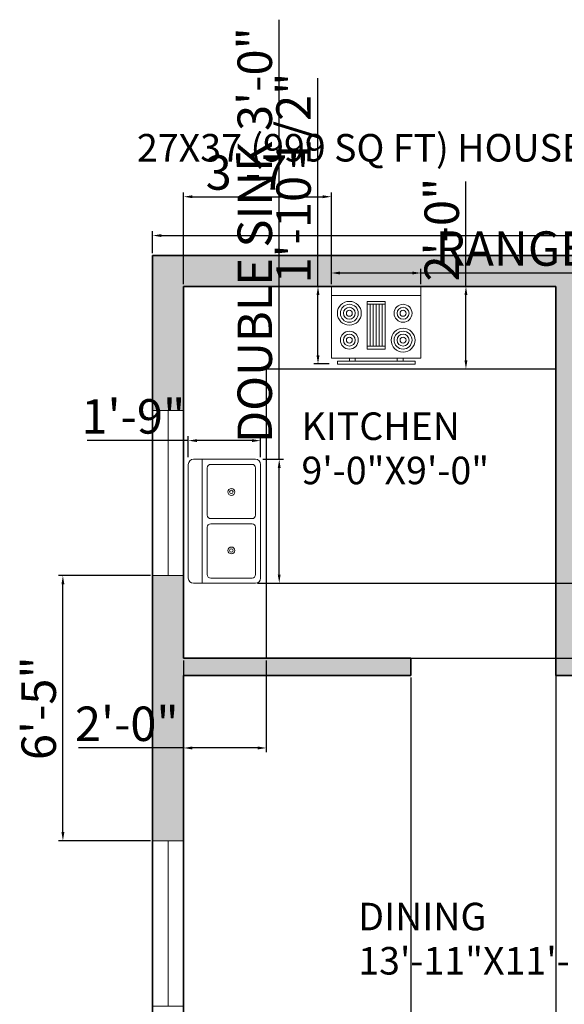
# Model space of a CAD drawing. Units: inches. Extents: x 3647 to 4124, y 1633 to 2205.
# Tile 2 of 3: x 3675 to 3833, y 1919 to 2205. Entities that reach past the tile are written whole.
import ezdxf

# ---------------------------------------------------------------- set-up
doc = ezdxf.new("R2010")
doc.units = ezdxf.units.IN
for name, color, linetype, lineweight in [('A-ANNO-DIMS', 2, 'Continuous', 18), ('A-ANNO-TEXT', 3, 'Continuous', 25), ('A-AREA-IDEN', 3, 'Continuous', 18), ('A-EQPM', 8, 'Continuous', 18), ('A-FLOR-CASE', 32, 'Continuous', 25), ('A-FLOR-FIXT', 9, 'Continuous', 18), ('WALL', 42, 'Continuous', 35), ('WINDOW', 4, 'Continuous', 18)]:
    doc.layers.add(name, color=color, linetype=linetype, lineweight=lineweight)
doc.layers.add('A-WALL-PATT', color=18, linetype='Continuous', lineweight=13, true_color=0x000000)
doc.styles.get("Standard").update_dxf_attribs({"font": 'arial.ttf'})
doc.dimstyles.new('ISO-25', dxfattribs={"dimtxt": 10, "dimasz": 2.5, "dimexe": 1.25, "dimexo": 0.625, "dimtad": 1, "dimdec": 1, "dimlunit": 3, "dimtxsty": 'Standard', "dimcen": 2.5, "dimadec": 0, "dimazin": 0, "dimtfac": 1, "dimtdec": 1, "dimtmove": 0, "dimatfit": 3, "dimfxl": 1, "dimarcsym": 0})

# ---------------------------------------------------------------- blocks, each defined once
blk = doc.blocks.new('Range-Oven - 30 in top')
for p, q in [((0, -3), (30, -3)), ((12, -6), (18, -6)), ((13, -20), (13, -6)), ((14, -6), (14, -20)), ((15, -20), (15, -6)), ((16, -6), (16, -20)), ((17, -20), (17, -6)), ((18, -20), (12, -20)), ((6, -24), (6, -25)), ((8, -25), (8, -24)), ((22, -25), (22, -24)), ((24, -24), (24, -25))]:
    blk.add_line(p, q)
for points in [[(0, -24), (0, 0), (30, 0), (30, -24)], [(12, -21), (12, -5), (18, -5), (18, -21)], [(2, -26), (2, -25), (28, -25), (28, -26)]]:
    blk.add_lwpolyline(points, close=True)
for centre, radius in [((6, -9), 4), ((6, -9), 3), ((24, -9), 3), ((6, -9), 2), ((6, -9), 1), ((24, -9), 2), ((24, -9), 1), ((6, -18), 3), ((6, -18), 2), ((24, -18), 4), ((24, -18), 3), ((24, -18), 2), ((6, -18), 1), ((24, -18), 1)]:
    blk.add_circle(centre, radius)
blk = doc.blocks.new('Sink-double - 36 in top')
for p, q in [((-18, -4), (18, -4)), ((-0.75, -18.5), (-0.75, -6.5)), ((0.75, -6.5), (0.75, -18.5))]:
    blk.add_line(p, q)
for points in [[(-16.5, 0), (16.5, 0)], [(-18, -19.5), (-18, -1.5)], [(18, -1.5), (18, -19.5)], [(-15.5, -5.5), (-1.75, -5.5)], [(1.75, -5.5), (15.5, -5.5)], [(-16.5, -18.5), (-16.5, -6.5)], [(16.5, -6.5), (16.5, -18.5)], [(-1.75, -19.5), (-15.5, -19.5)], [(15.5, -19.5), (1.75, -19.5)], [(16.5, -21), (-16.5, -21)]]:
    blk.add_lwpolyline(points)
for centre, radius in [((-8.5, -12.5), 1), ((-8.5, -12.5), 0.5), ((8.5, -12.5), 1), ((8.5, -12.5), 0.5)]:
    blk.add_circle(centre, radius)
for centre, radius, start, end in [((-16.5, -1.5), 1.5, 90, 180), ((16.5, -1.5), 1.5, 0, 90), ((-15.5, -6.5), 1, 90, 180), ((-1.75, -6.5), 1, 0, 90), ((1.75, -6.5), 1, 90, 180), ((15.5, -6.5), 1, 0, 90), ((-16.5, -19.5), 1.5, 180, 270), ((-15.5, -18.5), 1, 180, 270), ((-1.75, -18.5), 1, 270, 0), ((1.75, -18.5), 1, 180, 270), ((15.5, -18.5), 1, 270, 0), ((16.5, -19.5), 1.5, 270, 0)]:
    blk.add_arc(centre, radius, start, end)
blk = doc.blocks.new('*D11')
at = {"layer": 'A-ANNO-DIMS', "color": 0, "lineweight": -2, "transparency": 16777216}
for p, q in [((3713.71, 2136.91), (3713.71, 2143.3)), ((3716.21, 2142.05), (4035.21, 2142.05)), ((4037.71, 2136.91), (4037.71, 2143.3))]:
    blk.add_line(p, q, dxfattribs=at)
at = {"layer": 'A-ANNO-DIMS', "color": 0, "transparency": 16777216}
for points in [[(3716.21, 2142.46), (3716.21, 2141.63), (3713.71, 2142.05)], [(4035.21, 2142.46), (4035.21, 2141.63), (4037.71, 2142.05)]]:
    blk.add_solid(points, dxfattribs=at)
at = {"layer": 'Defpoints', "color": 0, "transparency": 16777216}
for p in [(4037.71, 2142.05), (3713.71, 2136.28), (4037.71, 2136.28)]:
    blk.add_point(p, dxfattribs=at)
at = {"layer": 'A-ANNO-DIMS', "color": 0, "transparency": 16777216, "insert": (3875.71, 2147.69), "char_height": 10, "attachment_point": 5}
blk.add_mtext("27'", dxfattribs=at)
blk = doc.blocks.new('WIN-48IN')
for p, q in [((9, 48), (0, 48)), ((4.5, 48), (4.5, 0)), ((9, 0), (0, 0))]:
    blk.add_line(p, q)
blk = doc.blocks.new('*D21')
at = {"layer": 'A-ANNO-DIMS', "color": 0, "lineweight": -2, "transparency": 16777216}
for p, q in [((3765.61, 2127.91), (3765.61, 2132.43)), ((3768.11, 2131.18), (3789.11, 2131.18)), ((3791.61, 2127.91), (3791.61, 2132.43)), ((3791.61, 2131.18), (3874.98, 2131.18))]:
    blk.add_line(p, q, dxfattribs=at)
at = {"layer": 'A-ANNO-DIMS', "color": 0, "transparency": 16777216}
for points in [[(3768.11, 2131.6), (3768.11, 2130.76), (3765.61, 2131.18)], [(3789.11, 2131.6), (3789.11, 2130.76), (3791.61, 2131.18)]]:
    blk.add_solid(points, dxfattribs=at)
at = {"layer": 'Defpoints', "color": 0, "transparency": 16777216}
for p in [(3791.61, 2131.18), (3765.61, 2127.28), (3791.61, 2127.28)]:
    blk.add_point(p, dxfattribs=at)
at = {"layer": 'A-ANNO-DIMS', "color": 0, "transparency": 16777216, "insert": (3834.55, 2136.98), "char_height": 10, "attachment_point": 5}
blk.add_mtext('RANGE 2\'-2"', dxfattribs=at)
blk = doc.blocks.new('*D22')
at = {"layer": 'A-ANNO-DIMS', "color": 0, "lineweight": -2, "transparency": 16777216}
for p, q in [((3761.71, 2127.28), (3761.71, 2187.74)), ((3764.98, 2127.28), (3760.46, 2127.28)), ((3761.71, 2107.25), (3761.71, 2124.78)), ((3764.98, 2104.75), (3760.46, 2104.75))]:
    blk.add_line(p, q, dxfattribs=at)
at = {"layer": 'A-ANNO-DIMS', "color": 0, "transparency": 16777216}
for points in [[(3761.29, 2124.78), (3762.13, 2124.78), (3761.71, 2127.28)], [(3761.29, 2107.25), (3762.13, 2107.25), (3761.71, 2104.75)]]:
    blk.add_solid(points, dxfattribs=at)
at = {"layer": 'Defpoints', "color": 0, "transparency": 16777216}
for p in [(3761.71, 2127.28), (3765.61, 2127.28), (3765.61, 2104.75)]:
    blk.add_point(p, dxfattribs=at)
at = {"layer": 'A-ANNO-DIMS', "color": 0, "transparency": 16777216, "insert": (3755.91, 2158.76), "char_height": 10, "attachment_point": 5, "rotation": 90}
blk.add_mtext('1\'-10 1/2"', dxfattribs=at)
blk = doc.blocks.new('*D23')
at = {"layer": 'A-ANNO-DIMS', "color": 0, "lineweight": -2, "transparency": 16777216}
for p, q in [((3750.46, 2077.09), (3750.46, 2204.75)), ((3745.68, 2077.09), (3751.71, 2077.09)), ((3750.46, 2043.59), (3750.46, 2074.59)), ((3745.68, 2041.09), (3751.71, 2041.09))]:
    blk.add_line(p, q, dxfattribs=at)
at = {"layer": 'A-ANNO-DIMS', "color": 0, "transparency": 16777216}
for points in [[(3750.04, 2074.59), (3750.87, 2074.59), (3750.46, 2077.09)], [(3750.04, 2043.59), (3750.87, 2043.59), (3750.46, 2041.09)]]:
    blk.add_solid(points, dxfattribs=at)
at = {"layer": 'Defpoints', "color": 0, "transparency": 16777216}
for p in [(3745.06, 2077.09), (3750.46, 2077.09), (3745.06, 2041.09)]:
    blk.add_point(p, dxfattribs=at)
at = {"layer": 'A-ANNO-DIMS', "color": 0, "transparency": 16777216, "insert": (3744.65, 2142.17), "char_height": 10, "attachment_point": 5, "rotation": 90}
blk.add_mtext('DOUBLE SINK 3\'-0"', dxfattribs=at)
blk = doc.blocks.new('*D24')
at = {"layer": 'A-ANNO-DIMS', "color": 0, "lineweight": -2, "transparency": 16777216}
for p, q in [((3724.06, 2082.49), (3694.66, 2082.49)), ((3724.06, 2077.72), (3724.06, 2083.74)), ((3742.56, 2082.49), (3726.56, 2082.49)), ((3745.06, 2077.72), (3745.06, 2083.74))]:
    blk.add_line(p, q, dxfattribs=at)
at = {"layer": 'A-ANNO-DIMS', "color": 0, "transparency": 16777216}
for points in [[(3726.56, 2082.91), (3726.56, 2082.08), (3724.06, 2082.49)], [(3742.56, 2082.91), (3742.56, 2082.08), (3745.06, 2082.49)]]:
    blk.add_solid(points, dxfattribs=at)
at = {"layer": 'Defpoints', "color": 0, "transparency": 16777216}
for p in [(3724.06, 2082.49), (3724.06, 2077.09), (3745.06, 2077.09)]:
    blk.add_point(p, dxfattribs=at)
at = {"layer": 'A-ANNO-DIMS', "color": 0, "transparency": 16777216, "insert": (3708.11, 2088.23), "char_height": 10, "attachment_point": 5}
blk.add_mtext('1\'-9"', dxfattribs=at)
blk = doc.blocks.new('*D31')
at = {"layer": 'A-ANNO-DIMS', "color": 0, "lineweight": -2, "transparency": 16777216}
for p, q in [((3788.71, 2013.66), (3788.71, 1644.98)), ((3830.71, 2013.66), (3830.71, 1644.98)), ((3791.21, 1646.23), (3828.21, 1646.23))]:
    blk.add_line(p, q, dxfattribs=at)
at = {"layer": 'A-ANNO-DIMS', "color": 0, "transparency": 16777216}
for points in [[(3791.21, 1646.65), (3791.21, 1645.81), (3788.71, 1646.23)], [(3828.21, 1646.65), (3828.21, 1645.81), (3830.71, 1646.23)]]:
    blk.add_solid(points, dxfattribs=at)
at = {"layer": 'Defpoints', "color": 0, "transparency": 16777216}
for p in [(3788.71, 2014.28), (3830.71, 2014.28), (3830.71, 1646.23)]:
    blk.add_point(p, dxfattribs=at)
at = {"layer": 'A-ANNO-DIMS', "color": 0, "transparency": 16777216, "insert": (3809.71, 1651.97), "char_height": 10, "attachment_point": 5}
blk.add_mtext('3\'-6"', dxfattribs=at)
blk = doc.blocks.new('*D32')
at = {"layer": 'A-ANNO-DIMS', "color": 0, "lineweight": -2, "transparency": 16777216}
for p, q in [((3830.71, 2126.66), (3830.71, 1644.98)), ((3835.71, 2126.66), (3835.71, 1644.98)), ((3828.21, 1646.23), (3825.71, 1646.23)), ((3830.71, 1646.23), (3835.71, 1646.23)), ((3838.21, 1646.23), (3868.55, 1646.23))]:
    blk.add_line(p, q, dxfattribs=at)
at = {"layer": 'A-ANNO-DIMS', "color": 0, "transparency": 16777216}
for points in [[(3828.21, 1646.65), (3828.21, 1645.81), (3830.71, 1646.23)], [(3838.21, 1646.65), (3838.21, 1645.81), (3835.71, 1646.23)]]:
    blk.add_solid(points, dxfattribs=at)
at = {"layer": 'Defpoints', "color": 0, "transparency": 16777216}
for p in [(3830.71, 2127.28), (3835.71, 2127.28), (3835.71, 1646.23)]:
    blk.add_point(p, dxfattribs=at)
at = {"layer": 'A-ANNO-DIMS', "color": 0, "transparency": 16777216, "insert": (3854.63, 1651.96), "char_height": 10, "attachment_point": 5}
blk.add_mtext('0\'-5"', dxfattribs=at)
blk = doc.blocks.new('*D40')
at = {"layer": 'A-ANNO-DIMS', "color": 0, "lineweight": -2, "transparency": 16777216}
for p, q in [((3713.09, 2043.28), (3686.41, 2043.28)), ((3687.66, 1968.78), (3687.66, 2040.78)), ((3713.09, 1966.28), (3686.41, 1966.28))]:
    blk.add_line(p, q, dxfattribs=at)
at = {"layer": 'A-ANNO-DIMS', "color": 0, "transparency": 16777216}
for points in [[(3687.25, 2040.78), (3688.08, 2040.78), (3687.66, 2043.28)], [(3687.25, 1968.78), (3688.08, 1968.78), (3687.66, 1966.28)]]:
    blk.add_solid(points, dxfattribs=at)
at = {"layer": 'Defpoints', "color": 0, "transparency": 16777216}
for p in [(3687.66, 2043.28), (3713.71, 2043.28), (3713.71, 1966.28)]:
    blk.add_point(p, dxfattribs=at)
at = {"layer": 'A-ANNO-DIMS', "color": 0, "transparency": 16777216, "insert": (3681.93, 2004.78), "char_height": 10, "attachment_point": 5, "rotation": 90}
blk.add_mtext('6\'-5"', dxfattribs=at)
blk = doc.blocks.new('*D52')
at = {"layer": 'A-ANNO-DIMS', "color": 0, "lineweight": -2, "transparency": 16777216}
for p, q in [((3722.71, 2018.66), (3722.71, 1991.98)), ((3746.71, 2018.66), (3746.71, 1991.98)), ((3722.71, 1993.23), (3692.21, 1993.23)), ((3744.21, 1993.23), (3725.21, 1993.23))]:
    blk.add_line(p, q, dxfattribs=at)
at = {"layer": 'A-ANNO-DIMS', "color": 0, "transparency": 16777216}
for points in [[(3725.21, 1993.65), (3725.21, 1992.81), (3722.71, 1993.23)], [(3744.21, 1993.65), (3744.21, 1992.81), (3746.71, 1993.23)]]:
    blk.add_solid(points, dxfattribs=at)
at = {"layer": 'Defpoints', "color": 0, "transparency": 16777216}
for p in [(3722.71, 2019.28), (3746.71, 2019.28), (3722.71, 1993.23)]:
    blk.add_point(p, dxfattribs=at)
at = {"layer": 'A-ANNO-DIMS', "color": 0, "transparency": 16777216, "insert": (3706.21, 1998.96), "char_height": 10, "attachment_point": 5}
blk.add_mtext('2\'-0"', dxfattribs=at)
blk = doc.blocks.new('*D53')
at = {"layer": 'A-ANNO-DIMS', "color": 0, "lineweight": -2, "transparency": 16777216}
for p, q in [((3804.66, 2127.28), (3804.66, 2157.78)), ((3830.09, 2127.28), (3803.41, 2127.28)), ((3804.66, 2105.78), (3804.66, 2124.78)), ((3830.09, 2103.28), (3803.41, 2103.28))]:
    blk.add_line(p, q, dxfattribs=at)
at = {"layer": 'A-ANNO-DIMS', "color": 0, "transparency": 16777216}
for points in [[(3804.25, 2124.78), (3805.08, 2124.78), (3804.66, 2127.28)], [(3804.25, 2105.78), (3805.08, 2105.78), (3804.66, 2103.28)]]:
    blk.add_solid(points, dxfattribs=at)
at = {"layer": 'Defpoints', "color": 0, "transparency": 16777216}
for p in [(3804.66, 2127.28), (3830.71, 2127.28), (3830.71, 2103.28)]:
    blk.add_point(p, dxfattribs=at)
at = {"layer": 'A-ANNO-DIMS', "color": 0, "transparency": 16777216, "insert": (3798.93, 2143.78), "char_height": 10, "attachment_point": 5, "rotation": 90}
blk.add_mtext('2\'-0"', dxfattribs=at)
blk = doc.blocks.new('*D54')
at = {"layer": 'A-ANNO-DIMS', "color": 0, "lineweight": -2, "transparency": 16777216}
for p, q in [((3722.71, 2127.91), (3722.71, 2154.58)), ((3725.21, 2153.33), (3763.11, 2153.33)), ((3765.61, 2127.91), (3765.61, 2154.58))]:
    blk.add_line(p, q, dxfattribs=at)
at = {"layer": 'A-ANNO-DIMS', "color": 0, "transparency": 16777216}
for points in [[(3725.21, 2153.75), (3725.21, 2152.91), (3722.71, 2153.33)], [(3763.11, 2153.75), (3763.11, 2152.91), (3765.61, 2153.33)]]:
    blk.add_solid(points, dxfattribs=at)
at = {"layer": 'Defpoints', "color": 0, "transparency": 16777216}
for p in [(3765.61, 2153.33), (3722.71, 2127.28), (3765.61, 2127.28)]:
    blk.add_point(p, dxfattribs=at)
at = {"layer": 'A-ANNO-DIMS', "color": 0, "transparency": 16777216, "insert": (3744.16, 2159.07), "char_height": 10, "attachment_point": 5}
blk.add_mtext('3\'-7"', dxfattribs=at)
blk = doc.blocks.new('*D55')
at = {"layer": 'A-ANNO-DIMS', "color": 0, "lineweight": -2, "transparency": 16777216}
for p, q in [((4114.76, 2041.09), (4114.76, 2078.26)), ((3744.18, 2041.09), (4116.01, 2041.09)), ((4114.76, 2021.78), (4114.76, 2038.59)), ((3747.34, 2019.28), (4116.01, 2019.28))]:
    blk.add_line(p, q, dxfattribs=at)
at = {"layer": 'A-ANNO-DIMS', "color": 0, "transparency": 16777216}
for points in [[(4114.35, 2038.59), (4115.18, 2038.59), (4114.76, 2041.09)], [(4114.35, 2021.78), (4115.18, 2021.78), (4114.76, 2019.28)]]:
    blk.add_solid(points, dxfattribs=at)
at = {"layer": 'Defpoints', "color": 0, "transparency": 16777216}
for p in [(3743.56, 2041.09), (4114.76, 2041.09), (3746.71, 2019.28)]:
    blk.add_point(p, dxfattribs=at)
at = {"layer": 'A-ANNO-DIMS', "color": 0, "transparency": 16777216, "insert": (4109.03, 2060.92), "char_height": 10, "attachment_point": 5, "rotation": 90}
blk.add_mtext('1\'-10"', dxfattribs=at)

msp = doc.modelspace()

# ---------------------------------------------------------------- hatches: boundary and pattern name
at = {"layer": 'A-WALL-PATT'}
h = msp.add_hatch(color=256, dxfattribs=at)
h.dxf.hatch_style = 1
h.paths.add_polyline_path([(3847.71, 2136.28), (3713.71, 2136.28), (3713.71, 2091.28), (3722.71, 2091.28), (3722.71, 2127.28), (3830.71, 2127.28), (3830.71, 2014.28), (3835.71, 2014.28), (3835.71, 2043.28), (3889.71, 2043.28), (3889.71, 2037.28), (3894.71, 2037.28), (3894.71, 2127.28), (4028.71, 2127.28), (4028.71, 2085.28), (4037.71, 2085.28), (4037.71, 2136.28), (3871.71, 2136.28), (3871.71, 2127.28), (3889.71, 2127.28), (3889.71, 2048.28), (3835.71, 2048.28), (3835.71, 2127.28), (3847.71, 2127.28)])
h.paths.add_polyline_path([(3839.02, 2091.4), (3895.07, 2091.4), (3895.07, 2103.66), (3839.02, 2103.66)], flags=25)
h = msp.add_hatch(color=256, dxfattribs=at)
h.dxf.hatch_style = 1
h.paths.add_polyline_path([(3722.71, 2014.28), (3788.71, 2014.28), (3788.71, 2019.28), (3722.71, 2019.28), (3722.71, 2043.28), (3713.71, 2043.28), (3713.71, 1966.28), (3722.71, 1966.28)])

# ---------------------------------------------------------------- linework, layer by layer
at = {"layer": 'A-FLOR-CASE'}
for p, q in [((3830.71, 2103.28), (3746.71, 2103.28)), ((3746.71, 2103.28), (3746.71, 2019.28))]:
    msp.add_line(p, q, dxfattribs=at)
at = {"layer": 'WALL'}
for p, q in [((3713.71, 2136.28), (4037.71, 2136.28)), ((3713.71, 1692.28), (3713.71, 2136.28)), ((3722.71, 2127.28), (3830.71, 2127.28)), ((3722.71, 2019.28), (3722.71, 2127.28)), ((3830.71, 2014.28), (3830.71, 2127.28)), ((3722.71, 2019.28), (3788.71, 2019.28)), ((3788.71, 2014.28), (3788.71, 2019.28)), ((3722.71, 2014.28), (3788.71, 2014.28)), ((3722.71, 1876.28), (3722.71, 2014.28)), ((3830.71, 2014.28), (3835.71, 2014.28))]:
    msp.add_line(p, q, dxfattribs=at)

# ---------------------------------------------------------------- block references
at = {"layer": 'A-EQPM', "xscale": 0.8666666666666667, "yscale": 0.8666666666666667, "zscale": 0.8666666666666667}
msp.add_blockref('Range-Oven - 30 in top', (3765.61, 2127.28), dxfattribs=at)
at = {"layer": 'A-FLOR-FIXT', "rotation": 90}
msp.add_blockref('Sink-double - 36 in top', (3724.06, 2059.09), dxfattribs=at)
at = {"layer": 'WINDOW', "rotation": 180}
msp.add_blockref('WIN-48IN', (3722.71, 2091.28), dxfattribs=at)
at = {"layer": 'WINDOW'}
msp.add_blockref('WIN-48IN', (3713.71, 1918.28), dxfattribs=at)

# ---------------------------------------------------------------- texts
at = {"layer": 'A-ANNO-TEXT'}
msp.add_text('27X37 (999 SQ FT) HOUSE PLAN -NORTH FACE-FP1071', height=8, dxfattribs=at).set_placement((3709.15, 2163.55))
at = {"layer": 'A-AREA-IDEN'}
for s, p in [('KITCHEN', (3756.91, 2082.68)), ('9\'-0"X9\'-0"', (3756.91, 2069.83)), ('DINING', (3773.39, 1940.27)), ('13\'-11"X11\'-6"', (3773.39, 1927.42))]:
    msp.add_text(s, height=8, dxfattribs=at).set_placement(p)

# ---------------------------------------------------------------- dimensions: what is measured, and where the dimension line sits
at = {"layer": 'A-ANNO-DIMS'}
dim = msp.add_linear_dim(base=(3750.46, 2077.09), p1=(3745.06, 2041.09), p2=(3745.06, 2077.09), angle=90, text='DOUBLE SINK <>', dimstyle='ISO-25', override={"dimdec": 1, "dimlfac": 1, "dimrnd": 0, "dimzin": 1, "dimdsep": 46, "dimlunit": 4, "dimfrac": 2}, dxfattribs=at)
dim.commit()
dim.dimension.update_dxf_attribs({"geometry": '*D23', "text_midpoint": (3744.65, 2142.17)})
for base, p1, p2, angle, picture, middle in [((3761.71, 2127.28), (3765.61, 2104.75), (3765.61, 2127.28), 90, '*D22', (3755.91, 2158.76)), ((3804.66, 2127.28), (3830.71, 2103.28), (3830.71, 2127.28), 90, '*D53', (3798.93, 2143.78)), ((3724.06, 2082.49), (3745.06, 2077.09), (3724.06, 2077.09), 180, '*D24', (3708.11, 2088.23)), ((4114.76, 2041.09), (3746.71, 2019.28), (3743.56, 2041.09), 90, '*D55', (4109.03, 2060.92)), ((3687.66, 2043.28), (3713.71, 1966.28), (3713.71, 2043.28), 90, '*D40', (3681.93, 2004.78)), ((3722.71, 1993.23), (3746.71, 2019.28), (3722.71, 2019.28), 180, '*D52', (3706.21, 1998.96))]:
    dim = msp.add_linear_dim(base=base, p1=p1, p2=p2, angle=angle, dimstyle='ISO-25', override={"dimdec": 1, "dimlfac": 1, "dimrnd": 0, "dimzin": 1, "dimdsep": 46, "dimlunit": 4, "dimfrac": 2}, dxfattribs=at)
    dim.commit()
    dim.dimension.update_dxf_attribs({"geometry": picture, "text_midpoint": middle})
for base, p1, p2, override, picture, middle in [((3765.61, 2153.33), (3722.71, 2127.28), (3765.61, 2127.28), {"dimdec": 1, "dimlfac": 1, "dimrnd": 0, "dimzin": 1, "dimdsep": 46, "dimlunit": 4, "dimfrac": 2}, '*D54', (3744.16, 2159.07)), ((4037.71, 2142.05), (3713.71, 2136.28), (4037.71, 2136.28), {"dimclrd": 0, "dimclre": 0, "dimclrt": 0}, '*D11', (3875.71, 2147.69)), ((3835.71, 1646.23), (3830.71, 2127.28), (3835.71, 2127.28), {"dimdec": 1, "dimlfac": 1, "dimrnd": 0, "dimzin": 1, "dimdsep": 46, "dimlunit": 4, "dimfrac": 2}, '*D32', (3854.63, 1651.96)), ((3830.71, 1646.23), (3788.71, 2014.28), (3830.71, 2014.28), {"dimdec": 1, "dimlfac": 1, "dimrnd": 0, "dimzin": 1, "dimdsep": 46, "dimlunit": 4, "dimfrac": 2}, '*D31', (3809.71, 1651.97))]:
    dim = msp.add_linear_dim(base=base, p1=p1, p2=p2, dimstyle='ISO-25', override=override, dxfattribs=at)
    dim.commit()
    dim.dimension.update_dxf_attribs({"geometry": picture, "text_midpoint": middle})
dim = msp.add_linear_dim(base=(3791.61, 2131.18), p1=(3765.61, 2127.28), p2=(3791.61, 2127.28), text='RANGE <>', dimstyle='ISO-25', override={"dimdec": 1, "dimlfac": 1, "dimrnd": 0, "dimzin": 1, "dimdsep": 46, "dimlunit": 4, "dimfrac": 2}, dxfattribs=at)
dim.commit()
dim.dimension.update_dxf_attribs({"geometry": '*D21', "text_midpoint": (3834.55, 2136.98)})

doc.saveas('drawing.dxf')
